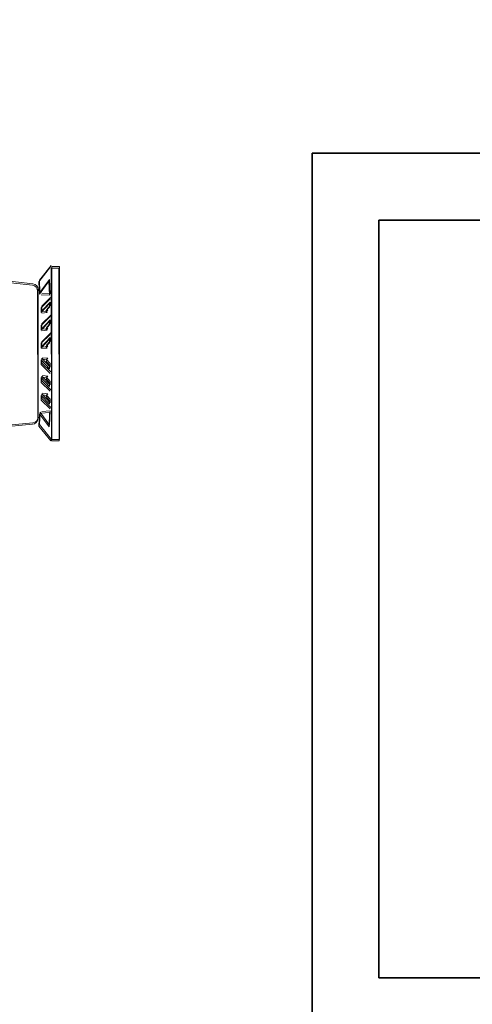
# Model space of a CAD drawing. Units: inches. Extents: x -26 to 575, y -18 to 513.
# Tile 22 of 28: x 355 to 385, y 241 to 307. Entities that reach past the tile are written whole.
import ezdxf

# ---------------------------------------------------------------- set-up
doc = ezdxf.new("R2010")
doc.units = ezdxf.units.IN
doc.header["$MEASUREMENT"] = 0
for name, color, linetype, lineweight in [('A-ANNO-DIMS', 2, 'Continuous', 18), ('A-WALL', 7, 'Continuous', 35), ('Furniture', 8, 'Continuous', 15)]:
    doc.layers.add(name, color=color, linetype=linetype, lineweight=lineweight)
doc.styles.get("Standard").update_dxf_attribs({"font": 'arial.ttf', "height": 6})
doc.dimstyles.get("Standard").update_dxf_attribs({"dimtxt": 6, "dimasz": 0.18, "dimexe": 0.18, "dimexo": 0.0625, "dimgap": 0.09, "dimtad": 0, "dimtih": 1, "dimtoh": 1, "dimzin": 0, "dimdsep": 46, "dimlunit": 3, "dimtxsty": 'Standard', "dimcen": 0.09, "dimadec": 0, "dimazin": 0, "dimtfac": 1, "dimtofl": 0, "dimtmove": 0, "dimatfit": 3, "dimfxl": 1, "dimtolj": 1, "dimtzin": 0, "dimarcsym": 0})

# ---------------------------------------------------------------- blocks, each defined once
blk = doc.blocks.new('DINING-SET-6-SEAT')
for p, q in [((16.828, 40.76, -3.573), (16.828, 41.278, -3.573)), ((16.828, 41.278, -3.573), (28.461, 41.278, -3.573)), ((16.931, 40.798, -3.573), (16.931, 41.316, -3.573)), ((16.931, 41.316, -3.573), (28.564, 41.316, -3.573)), ((28.461, 41.278, -3.573), (28.461, 40.76, -3.573)), ((28.564, 41.316, -3.573), (28.564, 40.798, -3.573)), ((47.187, 41.329, -3.573), (35.554, 41.319, -3.573)), ((35.554, 41.319, -3.573), (35.554, 40.801, -3.573)), ((47.29, 41.291, -3.573), (35.657, 41.281, -3.573)), ((35.657, 41.281, -3.573), (35.657, 40.763, -3.573)), ((47.188, 40.811, -3.573), (47.187, 41.329, -3.573)), ((47.29, 40.774, -3.573), (47.29, 41.291, -3.573)), ((28.461, 40.76, -3.573), (16.828, 40.76, -3.573)), ((16.828, 40.72, -3.573), (17.824, 39.924, -3.573)), ((28.564, 40.798, -3.573), (16.931, 40.798, -3.573)), ((16.931, 40.758, -3.573), (17.927, 39.962, -3.573)), ((17.784, 40.601, -3.573), (18.74, 40.641, -3.573)), ((18.661, 39.964, -3.573), (17.784, 40.601, -3.573)), ((17.887, 40.639, -3.573), (18.843, 40.679, -3.573)), ((18.763, 40.002, -3.573), (17.887, 40.639, -3.573)), ((18.74, 40.641, -3.573), (18.7, 40.083, -3.573)), ((18.843, 40.679, -3.573), (18.803, 40.121, -3.573)), ((18.979, 40.681, -3.573), (19.577, 40.083, -3.573)), ((19.082, 40.718, -3.573), (19.68, 40.121, -3.573)), ((19.896, 40.083, -3.573), (19.298, 40.641, -3.573)), ((19.298, 40.641, -3.573), (19.537, 40.641, -3.573)), ((19.998, 40.121, -3.573), (19.401, 40.679, -3.573)), ((19.401, 40.679, -3.573), (19.64, 40.679, -3.573)), ((19.537, 40.641, -3.573), (19.816, 40.402, -3.573)), ((19.64, 40.679, -3.573), (19.919, 40.44, -3.573)), ((19.816, 40.402, -3.573), (19.896, 40.481, -3.573)), ((19.896, 40.481, -3.573), (19.936, 40.123, -3.573)), ((19.919, 40.44, -3.573), (19.998, 40.519, -3.573)), ((19.998, 40.519, -3.573), (20.038, 40.161, -3.573)), ((20.175, 40.681, -3.573), (20.772, 40.083, -3.573)), ((20.277, 40.718, -3.573), (20.875, 40.121, -3.573)), ((21.091, 40.083, -3.573), (20.493, 40.641, -3.573)), ((20.493, 40.641, -3.573), (20.732, 40.641, -3.573)), ((21.194, 40.121, -3.573), (20.596, 40.679, -3.573)), ((20.596, 40.679, -3.573), (20.835, 40.679, -3.573)), ((20.732, 40.641, -3.573), (21.011, 40.402, -3.573)), ((20.835, 40.679, -3.573), (21.114, 40.44, -3.573)), ((21.011, 40.402, -3.573), (21.091, 40.481, -3.573)), ((21.091, 40.481, -3.573), (21.131, 40.123, -3.573)), ((21.114, 40.44, -3.573), (21.194, 40.519, -3.573)), ((21.194, 40.519, -3.573), (21.233, 40.161, -3.573)), ((21.37, 40.681, -3.573), (21.967, 40.083, -3.573)), ((21.473, 40.718, -3.573), (22.07, 40.121, -3.573)), ((22.286, 40.083, -3.573), (21.688, 40.641, -3.573)), ((21.688, 40.641, -3.573), (21.928, 40.641, -3.573)), ((22.389, 40.121, -3.573), (21.791, 40.679, -3.573)), ((21.791, 40.679, -3.573), (22.03, 40.679, -3.573)), ((21.928, 40.641, -3.573), (22.206, 40.402, -3.573)), ((22.03, 40.679, -3.573), (22.309, 40.44, -3.573)), ((22.206, 40.402, -3.573), (22.286, 40.481, -3.573)), ((22.286, 40.481, -3.573), (22.326, 40.123, -3.573)), ((22.309, 40.44, -3.573), (22.389, 40.519, -3.573)), ((22.389, 40.519, -3.573), (22.429, 40.161, -3.573)), ((23.083, 40.481, -3.573), (23.043, 40.123, -3.573)), ((23.083, 40.083, -3.573), (23.681, 40.641, -3.573)), ((23.163, 40.402, -3.573), (23.083, 40.481, -3.573)), ((23.186, 40.519, -3.573), (23.146, 40.161, -3.573)), ((23.441, 40.641, -3.573), (23.163, 40.402, -3.573)), ((23.186, 40.121, -3.573), (23.783, 40.679, -3.573)), ((23.265, 40.44, -3.573), (23.186, 40.519, -3.573)), ((23.544, 40.679, -3.573), (23.265, 40.44, -3.573)), ((23.999, 40.681, -3.573), (23.402, 40.083, -3.573)), ((23.681, 40.641, -3.573), (23.441, 40.641, -3.573)), ((24.102, 40.718, -3.573), (23.504, 40.121, -3.573)), ((23.783, 40.679, -3.573), (23.544, 40.679, -3.573)), ((24.278, 40.481, -3.573), (24.238, 40.123, -3.573)), ((24.278, 40.083, -3.573), (24.876, 40.641, -3.573)), ((24.358, 40.402, -3.573), (24.278, 40.481, -3.573)), ((24.381, 40.519, -3.573), (24.341, 40.161, -3.573)), ((24.637, 40.641, -3.573), (24.358, 40.402, -3.573)), ((24.381, 40.121, -3.573), (24.978, 40.679, -3.573)), ((24.461, 40.44, -3.573), (24.381, 40.519, -3.573)), ((24.739, 40.679, -3.573), (24.461, 40.44, -3.573)), ((25.194, 40.681, -3.573), (24.597, 40.083, -3.573)), ((24.876, 40.641, -3.573), (24.637, 40.641, -3.573)), ((25.297, 40.718, -3.573), (24.7, 40.121, -3.573)), ((24.978, 40.679, -3.573), (24.739, 40.679, -3.573)), ((25.473, 40.481, -3.573), (25.434, 40.123, -3.573)), ((25.473, 40.083, -3.573), (26.071, 40.641, -3.573)), ((25.553, 40.402, -3.573), (25.473, 40.481, -3.573)), ((25.576, 40.519, -3.573), (25.536, 40.161, -3.573)), ((25.832, 40.641, -3.573), (25.553, 40.402, -3.573)), ((25.576, 40.121, -3.573), (26.174, 40.679, -3.573)), ((25.656, 40.44, -3.573), (25.576, 40.519, -3.573)), ((25.935, 40.679, -3.573), (25.656, 40.44, -3.573)), ((26.39, 40.681, -3.573), (25.792, 40.083, -3.573)), ((26.071, 40.641, -3.573), (25.832, 40.641, -3.573)), ((26.492, 40.718, -3.573), (25.895, 40.121, -3.573)), ((26.174, 40.679, -3.573), (25.935, 40.679, -3.573)), ((27.585, 40.601, -3.573), (26.629, 40.641, -3.573)), ((26.629, 40.641, -3.573), (26.669, 40.083, -3.573)), ((26.708, 39.964, -3.573), (27.585, 40.601, -3.573)), ((27.688, 40.639, -3.573), (26.731, 40.679, -3.573)), ((26.731, 40.679, -3.573), (26.771, 40.121, -3.573)), ((26.811, 40.002, -3.573), (27.688, 40.639, -3.573)), ((28.541, 40.72, -3.573), (27.545, 39.924, -3.573)), ((28.644, 40.758, -3.573), (27.648, 39.962, -3.573)), ((35.475, 40.761, -3.573), (36.471, 39.966, -3.573)), ((35.554, 40.801, -3.573), (47.188, 40.811, -3.573)), ((35.577, 40.723, -3.573), (36.574, 39.928, -3.573)), ((35.657, 40.763, -3.573), (47.29, 40.774, -3.573)), ((36.431, 40.643, -3.573), (37.387, 40.683, -3.573)), ((37.308, 40.006, -3.573), (36.431, 40.643, -3.573)), ((36.534, 40.605, -3.573), (37.49, 40.646, -3.573)), ((37.411, 39.968, -3.573), (36.534, 40.605, -3.573)), ((37.387, 40.683, -3.573), (37.348, 40.126, -3.573)), ((37.49, 40.646, -3.573), (37.45, 40.088, -3.573)), ((37.626, 40.723, -3.573), (38.224, 40.127, -3.573)), ((37.729, 40.686, -3.573), (38.327, 40.089, -3.573)), ((38.543, 40.127, -3.573), (37.945, 40.684, -3.573)), ((37.945, 40.684, -3.573), (38.184, 40.684, -3.573)), ((38.646, 40.089, -3.573), (38.048, 40.646, -3.573)), ((38.048, 40.646, -3.573), (38.287, 40.646, -3.573)), ((38.184, 40.684, -3.573), (38.463, 40.445, -3.573)), ((38.287, 40.646, -3.573), (38.566, 40.408, -3.573)), ((38.463, 40.445, -3.573), (38.543, 40.525, -3.573)), ((38.543, 40.525, -3.573), (38.583, 40.167, -3.573)), ((38.566, 40.408, -3.573), (38.645, 40.487, -3.573)), ((38.645, 40.487, -3.573), (38.685, 40.129, -3.573)), ((38.821, 40.724, -3.573), (39.419, 40.128, -3.573)), ((38.924, 40.687, -3.573), (39.522, 40.09, -3.573)), ((39.738, 40.128, -3.573), (39.14, 40.685, -3.573)), ((39.14, 40.685, -3.573), (39.379, 40.685, -3.573)), ((39.841, 40.09, -3.573), (39.243, 40.647, -3.573)), ((39.243, 40.647, -3.573), (39.482, 40.647, -3.573)), ((39.379, 40.685, -3.573), (39.658, 40.446, -3.573)), ((39.482, 40.647, -3.573), (39.761, 40.409, -3.573)), ((39.658, 40.446, -3.573), (39.738, 40.526, -3.573)), ((39.738, 40.526, -3.573), (39.778, 40.168, -3.573)), ((39.761, 40.409, -3.573), (39.841, 40.488, -3.573)), ((39.841, 40.488, -3.573), (39.881, 40.13, -3.573)), ((40.016, 40.725, -3.573), (40.615, 40.129, -3.573)), ((40.119, 40.688, -3.573), (40.717, 40.091, -3.573)), ((40.933, 40.129, -3.573), (40.335, 40.686, -3.573)), ((40.335, 40.686, -3.573), (40.574, 40.686, -3.573)), ((41.036, 40.091, -3.573), (40.438, 40.648, -3.573)), ((40.438, 40.648, -3.573), (40.677, 40.648, -3.573)), ((40.574, 40.686, -3.573), (40.853, 40.447, -3.573)), ((40.677, 40.648, -3.573), (40.956, 40.41, -3.573)), ((40.853, 40.447, -3.573), (40.933, 40.527, -3.573)), ((40.933, 40.527, -3.573), (40.973, 40.169, -3.573)), ((40.956, 40.41, -3.573), (41.036, 40.489, -3.573)), ((41.036, 40.489, -3.573), (41.076, 40.131, -3.573)), ((41.73, 40.528, -3.573), (41.69, 40.169, -3.573)), ((41.73, 40.13, -3.573), (42.327, 40.688, -3.573)), ((41.81, 40.448, -3.573), (41.73, 40.528, -3.573)), ((41.833, 40.49, -3.573), (41.793, 40.132, -3.573)), ((42.088, 40.687, -3.573), (41.81, 40.448, -3.573)), ((41.833, 40.092, -3.573), (42.43, 40.65, -3.573)), ((41.912, 40.41, -3.573), (41.833, 40.49, -3.573)), ((42.191, 40.65, -3.573), (41.912, 40.41, -3.573)), ((42.646, 40.728, -3.573), (42.049, 40.13, -3.573)), ((42.327, 40.688, -3.573), (42.088, 40.687, -3.573)), ((42.749, 40.69, -3.573), (42.152, 40.092, -3.573)), ((42.43, 40.65, -3.573), (42.191, 40.65, -3.573)), ((42.925, 40.529, -3.573), (42.885, 40.17, -3.573)), ((42.925, 40.131, -3.573), (43.522, 40.689, -3.573)), ((43.005, 40.449, -3.573), (42.925, 40.529, -3.573)), ((43.028, 40.491, -3.573), (42.988, 40.133, -3.573)), ((43.283, 40.688, -3.573), (43.005, 40.449, -3.573)), ((43.028, 40.093, -3.573), (43.625, 40.651, -3.573)), ((43.108, 40.412, -3.573), (43.028, 40.491, -3.573)), ((43.386, 40.651, -3.573), (43.108, 40.412, -3.573)), ((43.841, 40.729, -3.573), (43.244, 40.131, -3.573)), ((43.522, 40.689, -3.573), (43.283, 40.688, -3.573)), ((43.944, 40.691, -3.573), (43.347, 40.093, -3.573)), ((43.625, 40.651, -3.573), (43.386, 40.651, -3.573)), ((44.12, 40.53, -3.573), (44.081, 40.171, -3.573)), ((44.2, 40.45, -3.573), (44.12, 40.53, -3.573)), ((44.121, 40.132, -3.573), (44.718, 40.69, -3.573)), ((44.223, 40.492, -3.573), (44.183, 40.134, -3.573)), ((44.479, 40.69, -3.573), (44.2, 40.45, -3.573)), ((44.223, 40.094, -3.573), (44.82, 40.652, -3.573)), ((44.303, 40.413, -3.573), (44.223, 40.492, -3.573)), ((44.581, 40.652, -3.573), (44.303, 40.413, -3.573)), ((45.036, 40.73, -3.573), (44.439, 40.132, -3.573)), ((44.718, 40.69, -3.573), (44.479, 40.69, -3.573)), ((45.139, 40.692, -3.573), (44.542, 40.094, -3.573)), ((44.82, 40.652, -3.573), (44.581, 40.652, -3.573)), ((46.232, 40.651, -3.573), (45.275, 40.69, -3.573)), ((45.275, 40.69, -3.573), (45.316, 40.133, -3.573)), ((45.356, 40.013, -3.573), (46.232, 40.651, -3.573)), ((46.334, 40.613, -3.573), (45.378, 40.652, -3.573)), ((45.378, 40.652, -3.573), (45.419, 40.095, -3.573)), ((45.458, 39.976, -3.573), (46.334, 40.613, -3.573)), ((47.188, 40.772, -3.573), (46.192, 39.974, -3.573)), ((47.29, 40.734, -3.573), (46.295, 39.936, -3.573)), ((17.824, 39.924, -3.573), (18.661, 39.964, -3.573)), ((17.927, 39.962, -3.573), (18.763, 40.002, -3.573)), ((26.909, 39.844, -3.573), (18.345, 39.844, -3.573)), ((27.012, 39.882, -3.573), (18.448, 39.882, -3.573)), ((19.577, 40.083, -3.573), (19.896, 40.083, -3.573)), ((19.68, 40.121, -3.573), (19.998, 40.121, -3.573)), ((20.772, 40.083, -3.573), (21.091, 40.083, -3.573)), ((20.875, 40.121, -3.573), (21.194, 40.121, -3.573)), ((21.967, 40.083, -3.573), (22.286, 40.083, -3.573)), ((22.07, 40.121, -3.573), (22.389, 40.121, -3.573)), ((23.402, 40.083, -3.573), (23.083, 40.083, -3.573)), ((23.504, 40.121, -3.573), (23.186, 40.121, -3.573)), ((24.597, 40.083, -3.573), (24.278, 40.083, -3.573)), ((24.7, 40.121, -3.573), (24.381, 40.121, -3.573)), ((25.792, 40.083, -3.573), (25.473, 40.083, -3.573)), ((25.895, 40.121, -3.573), (25.576, 40.121, -3.573)), ((27.545, 39.924, -3.573), (26.708, 39.964, -3.573)), ((27.648, 39.962, -3.573), (26.811, 40.002, -3.573)), ((36.471, 39.966, -3.573), (37.308, 40.006, -3.573)), ((36.574, 39.928, -3.573), (37.411, 39.968, -3.573)), ((37.107, 39.887, -3.573), (45.671, 39.894, -3.573)), ((37.21, 39.849, -3.573), (45.774, 39.856, -3.573)), ((38.224, 40.127, -3.573), (38.543, 40.127, -3.573)), ((38.327, 40.089, -3.573), (38.646, 40.089, -3.573)), ((39.419, 40.128, -3.573), (39.738, 40.128, -3.573)), ((39.522, 40.09, -3.573), (39.841, 40.09, -3.573)), ((40.615, 40.129, -3.573), (40.933, 40.129, -3.573)), ((40.717, 40.091, -3.573), (41.036, 40.091, -3.573)), ((42.049, 40.13, -3.573), (41.73, 40.13, -3.573)), ((42.152, 40.092, -3.573), (41.833, 40.092, -3.573)), ((43.244, 40.131, -3.573), (42.925, 40.131, -3.573)), ((43.347, 40.093, -3.573), (43.028, 40.093, -3.573)), ((44.439, 40.132, -3.573), (44.121, 40.132, -3.573)), ((44.542, 40.094, -3.573), (44.223, 40.094, -3.573)), ((46.192, 39.974, -3.573), (45.356, 40.013, -3.573)), ((46.295, 39.936, -3.573), (45.458, 39.976, -3.573)), ((17.949, 39.484, -3.573), (16.91, 28.653, -3.573)), ((18.052, 39.522, -3.573), (17.012, 28.691, -3.573)), ((28.493, 28.659, -3.573), (27.305, 39.489, -3.573)), ((28.595, 28.696, -3.573), (27.408, 39.527, -3.573)), ((35.534, 28.7, -3.573), (36.712, 39.531, -3.573)), ((35.636, 28.662, -3.573), (36.814, 39.494, -3.573)), ((46.068, 39.534, -3.573), (47.117, 28.704, -3.573)), ((46.171, 39.496, -3.573), (47.219, 28.667, -3.573)), ((16.194, 22.294, -1.308), (26.662, 30.717, -1.308)), ((46.474, 31.041, -1.308), (18.1, 31.041, -1.308)), ((14.74, 19.68, -1.308), (28.116, 30.426, -1.308)), ((25.79, 15.904, -1.308), (43.819, 30.136, -1.308)), ((17.306, 28.217, -3.573), (28.097, 28.217, -3.573)), ((17.409, 28.255, -3.573), (28.199, 28.255, -3.573)), ((46.72, 28.268, -3.573), (35.93, 28.258, -3.573)), ((46.823, 28.23, -3.573), (36.033, 28.22, -3.573)), ((18.1, 10.54, -1.308), (39.457, 27.522, -1.308)), ((0, 14.987, -3.573), (0.01, 26.621, -3.573)), ((0.01, 26.621, -3.573), (0.528, 26.62, -3.573)), ((0.037, 14.884, -3.573), (0.048, 26.518, -3.573)), ((0.048, 26.518, -3.573), (0.565, 26.517, -3.573)), ((0.528, 26.62, -3.573), (0.517, 14.987, -3.573)), ((0.565, 26.517, -3.573), (0.555, 14.884, -3.573)), ((0.567, 26.7, -3.573), (1.363, 25.703, -3.573)), ((0.605, 26.597, -3.573), (1.401, 25.6, -3.573)), ((12.629, 26.641, -3.573), (1.797, 25.463, -3.573)), ((12.667, 26.538, -3.573), (1.835, 25.36, -3.573)), ((52.057, 26.538, -3.573), (62.889, 25.36, -3.573)), ((52.095, 26.641, -3.573), (62.926, 25.463, -3.573)), ((64.119, 26.597, -3.573), (63.323, 25.6, -3.573)), ((64.156, 26.7, -3.573), (63.361, 25.703, -3.573)), ((64.676, 26.518, -3.573), (64.159, 26.517, -3.573)), ((64.159, 26.517, -3.573), (64.169, 14.884, -3.573)), ((64.714, 26.621, -3.573), (64.196, 26.62, -3.573)), ((64.196, 26.62, -3.573), (64.207, 14.987, -3.573)), ((64.686, 14.884, -3.573), (64.676, 26.518, -3.573)), ((64.724, 14.987, -3.573), (64.714, 26.621, -3.573)), ((13.061, 15.454, -3.573), (13.071, 26.244, -3.573)), ((13.099, 15.351, -3.573), (13.108, 26.142, -3.573)), ((51.625, 15.351, -3.573), (51.615, 26.142, -3.573)), ((51.663, 15.454, -3.573), (51.653, 26.244, -3.573)), ((0.686, 25.744, -3.573), (0.645, 24.787, -3.573)), ((0.724, 25.641, -3.573), (0.683, 24.685, -3.573)), ((1.322, 24.866, -3.573), (0.686, 25.744, -3.573)), ((1.36, 24.764, -3.573), (0.724, 25.641, -3.573)), ((1.363, 25.703, -3.573), (1.322, 24.866, -3.573)), ((1.401, 25.6, -3.573), (1.36, 24.764, -3.573)), ((63.323, 25.6, -3.573), (63.364, 24.764, -3.573)), ((63.361, 25.703, -3.573), (63.401, 24.866, -3.573)), ((63.364, 24.764, -3.573), (64, 25.641, -3.573)), ((63.401, 24.866, -3.573), (64.038, 25.744, -3.573)), ((64, 25.641, -3.573), (64.041, 24.685, -3.573)), ((64.038, 25.744, -3.573), (64.078, 24.787, -3.573)), ((0.605, 24.548, -3.573), (1.202, 23.95, -3.573)), ((0.645, 24.787, -3.573), (1.203, 24.827, -3.573)), ((0.683, 24.685, -3.573), (1.241, 24.724, -3.573)), ((1.442, 25.067, -3.573), (1.435, 16.503, -3.573)), ((1.48, 24.964, -3.573), (1.472, 16.401, -3.573)), ((63.244, 24.964, -3.573), (63.252, 16.401, -3.573)), ((63.282, 25.067, -3.573), (63.289, 16.503, -3.573)), ((64.041, 24.685, -3.573), (63.483, 24.724, -3.573)), ((64.078, 24.787, -3.573), (63.521, 24.827, -3.573)), ((64.118, 24.548, -3.573), (63.522, 23.95, -3.573)), ((0.643, 24.446, -3.573), (1.24, 23.847, -3.573)), ((1.202, 23.632, -3.573), (0.645, 24.23, -3.573)), ((0.645, 24.23, -3.573), (0.645, 23.991, -3.573)), ((0.645, 23.991, -3.573), (0.883, 23.712, -3.573)), ((0.683, 24.127, -3.573), (0.682, 23.888, -3.573)), ((0.682, 23.888, -3.573), (0.921, 23.609, -3.573)), ((1.24, 23.529, -3.573), (0.683, 24.127, -3.573)), ((1.202, 23.95, -3.573), (1.202, 23.632, -3.573)), ((40.039, 15.033, -1.308), (51.38, 24.327, -1.308)), ((64.081, 24.446, -3.573), (63.484, 23.847, -3.573)), ((63.484, 23.529, -3.573), (64.041, 24.127, -3.573)), ((63.522, 23.632, -3.573), (64.079, 24.23, -3.573)), ((63.522, 23.95, -3.573), (63.522, 23.632, -3.573)), ((64.041, 23.888, -3.573), (63.803, 23.609, -3.573)), ((64.079, 23.991, -3.573), (63.84, 23.712, -3.573)), ((64.041, 24.127, -3.573), (64.041, 23.888, -3.573)), ((64.079, 24.23, -3.573), (64.079, 23.991, -3.573)), ((0.604, 23.353, -3.573), (1.201, 22.755, -3.573)), ((0.642, 23.25, -3.573), (1.239, 22.652, -3.573)), ((0.883, 23.712, -3.573), (0.804, 23.632, -3.573)), ((0.804, 23.632, -3.573), (1.162, 23.592, -3.573)), ((0.921, 23.609, -3.573), (0.841, 23.529, -3.573)), ((0.841, 23.529, -3.573), (1.2, 23.489, -3.573)), ((1.24, 23.847, -3.573), (1.24, 23.529, -3.573)), ((63.484, 23.847, -3.573), (63.484, 23.529, -3.573)), ((64.082, 23.25, -3.573), (63.485, 22.652, -3.573)), ((64.12, 23.353, -3.573), (63.523, 22.755, -3.573)), ((63.882, 23.529, -3.573), (63.524, 23.489, -3.573)), ((63.92, 23.632, -3.573), (63.562, 23.592, -3.573)), ((63.803, 23.609, -3.573), (63.882, 23.529, -3.573)), ((63.84, 23.712, -3.573), (63.92, 23.632, -3.573)), ((1.201, 22.436, -3.573), (0.644, 23.034, -3.573)), ((0.644, 23.034, -3.573), (0.644, 22.795, -3.573)), ((0.644, 22.795, -3.573), (0.882, 22.516, -3.573)), ((0.682, 22.932, -3.573), (0.681, 22.693, -3.573)), ((0.681, 22.693, -3.573), (0.92, 22.414, -3.573)), ((1.239, 22.334, -3.573), (0.682, 22.932, -3.573)), ((1.201, 22.755, -3.573), (1.201, 22.436, -3.573)), ((1.239, 22.652, -3.573), (1.239, 22.334, -3.573)), ((63.485, 22.334, -3.573), (64.042, 22.932, -3.573)), ((63.485, 22.652, -3.573), (63.485, 22.334, -3.573)), ((63.523, 22.436, -3.573), (64.08, 23.034, -3.573)), ((63.523, 22.755, -3.573), (63.523, 22.436, -3.573)), ((64.042, 22.693, -3.573), (63.804, 22.414, -3.573)), ((64.08, 22.795, -3.573), (63.842, 22.516, -3.573)), ((64.042, 22.932, -3.573), (64.042, 22.693, -3.573)), ((64.08, 23.034, -3.573), (64.08, 22.795, -3.573)), ((0.603, 22.158, -3.573), (1.2, 21.56, -3.573)), ((0.641, 22.055, -3.573), (1.238, 21.457, -3.573)), ((0.882, 22.516, -3.573), (0.803, 22.437, -3.573)), ((0.803, 22.437, -3.573), (1.161, 22.397, -3.573)), ((0.92, 22.414, -3.573), (0.84, 22.334, -3.573)), ((0.84, 22.334, -3.573), (1.199, 22.294, -3.573)), ((64.083, 22.055, -3.573), (63.486, 21.457, -3.573)), ((64.121, 22.158, -3.573), (63.524, 21.56, -3.573)), ((63.883, 22.334, -3.573), (63.525, 22.294, -3.573)), ((63.921, 22.437, -3.573), (63.563, 22.397, -3.573)), ((63.804, 22.414, -3.573), (63.883, 22.334, -3.573)), ((63.842, 22.516, -3.573), (63.921, 22.437, -3.573)), ((1.2, 21.241, -3.573), (0.643, 21.839, -3.573)), ((0.643, 21.839, -3.573), (0.643, 21.6, -3.573)), ((0.643, 21.6, -3.573), (0.881, 21.321, -3.573)), ((0.681, 21.736, -3.573), (0.68, 21.497, -3.573)), ((0.68, 21.497, -3.573), (0.919, 21.218, -3.573)), ((1.238, 21.138, -3.573), (0.681, 21.736, -3.573)), ((0.881, 21.321, -3.573), (0.802, 21.241, -3.573)), ((0.802, 21.241, -3.573), (1.16, 21.201, -3.573)), ((0.919, 21.218, -3.573), (0.839, 21.139, -3.573)), ((1.2, 21.56, -3.573), (1.2, 21.241, -3.573)), ((1.238, 21.457, -3.573), (1.238, 21.138, -3.573)), ((63.486, 21.138, -3.573), (64.043, 21.736, -3.573)), ((63.486, 21.457, -3.573), (63.486, 21.138, -3.573)), ((63.524, 21.241, -3.573), (64.081, 21.839, -3.573)), ((63.524, 21.56, -3.573), (63.524, 21.241, -3.573)), ((63.922, 21.241, -3.573), (63.564, 21.201, -3.573)), ((64.043, 21.497, -3.573), (63.805, 21.218, -3.573)), ((63.805, 21.218, -3.573), (63.884, 21.139, -3.573)), ((64.081, 21.6, -3.573), (63.843, 21.321, -3.573)), ((63.843, 21.321, -3.573), (63.922, 21.241, -3.573)), ((64.043, 21.736, -3.573), (64.043, 21.497, -3.573)), ((64.081, 21.839, -3.573), (64.081, 21.6, -3.573)), ((0.839, 21.139, -3.573), (1.198, 21.099, -3.573)), ((63.884, 21.139, -3.573), (63.526, 21.099, -3.573)), ((0.601, 19.529, -3.573), (1.199, 20.126, -3.573)), ((0.639, 19.426, -3.573), (1.237, 20.023, -3.573)), ((1.199, 20.444, -3.573), (0.641, 19.847, -3.573)), ((0.641, 20.086, -3.573), (0.88, 20.365, -3.573)), ((0.641, 19.847, -3.573), (0.641, 20.086, -3.573)), ((1.237, 20.342, -3.573), (0.679, 19.744, -3.573)), ((0.679, 19.983, -3.573), (0.918, 20.262, -3.573)), ((0.679, 19.744, -3.573), (0.679, 19.983, -3.573)), ((0.801, 20.445, -3.573), (1.159, 20.484, -3.573)), ((0.88, 20.365, -3.573), (0.801, 20.445, -3.573)), ((0.839, 20.342, -3.573), (1.197, 20.381, -3.573)), ((0.918, 20.262, -3.573), (0.839, 20.342, -3.573)), ((1.199, 20.126, -3.573), (1.199, 20.444, -3.573)), ((1.237, 20.023, -3.573), (1.237, 20.342, -3.573)), ((34.805, 10.386, -1.308), (47.018, 19.971, -1.308)), ((63.487, 20.023, -3.573), (63.487, 20.342, -3.573)), ((63.487, 20.342, -3.573), (64.045, 19.744, -3.573)), ((64.085, 19.426, -3.573), (63.487, 20.023, -3.573)), ((63.525, 20.126, -3.573), (63.525, 20.444, -3.573)), ((63.525, 20.444, -3.573), (64.083, 19.847, -3.573)), ((64.123, 19.529, -3.573), (63.525, 20.126, -3.573)), ((63.885, 20.342, -3.573), (63.527, 20.381, -3.573)), ((63.923, 20.445, -3.573), (63.565, 20.484, -3.573)), ((63.806, 20.262, -3.573), (63.885, 20.342, -3.573)), ((64.045, 19.983, -3.573), (63.806, 20.262, -3.573)), ((63.843, 20.365, -3.573), (63.923, 20.445, -3.573)), ((64.083, 20.086, -3.573), (63.843, 20.365, -3.573)), ((64.045, 19.744, -3.573), (64.045, 19.983, -3.573)), ((64.083, 19.847, -3.573), (64.083, 20.086, -3.573)), ((1.198, 19.249, -3.573), (0.64, 18.652, -3.573)), ((0.8, 19.249, -3.573), (1.158, 19.289, -3.573)), ((0.879, 19.17, -3.573), (0.8, 19.249, -3.573)), ((1.198, 18.93, -3.573), (1.198, 19.249, -3.573)), ((63.526, 18.93, -3.573), (63.526, 19.249, -3.573)), ((63.526, 19.249, -3.573), (64.084, 18.652, -3.573)), ((63.924, 19.249, -3.573), (63.566, 19.289, -3.573)), ((63.844, 19.17, -3.573), (63.924, 19.249, -3.573)), ((0.6, 18.333, -3.573), (1.198, 18.93, -3.573)), ((0.638, 18.231, -3.573), (1.236, 18.828, -3.573)), ((0.64, 18.891, -3.573), (0.879, 19.17, -3.573)), ((0.64, 18.652, -3.573), (0.64, 18.891, -3.573)), ((1.236, 19.146, -3.573), (0.678, 18.549, -3.573)), ((0.678, 18.788, -3.573), (0.917, 19.067, -3.573)), ((0.678, 18.549, -3.573), (0.678, 18.788, -3.573)), ((0.838, 19.147, -3.573), (1.196, 19.186, -3.573)), ((0.917, 19.067, -3.573), (0.838, 19.147, -3.573)), ((1.236, 18.828, -3.573), (1.236, 19.146, -3.573)), ((63.488, 18.828, -3.573), (63.488, 19.146, -3.573)), ((63.488, 19.146, -3.573), (64.046, 18.549, -3.573)), ((64.086, 18.231, -3.573), (63.488, 18.828, -3.573)), ((64.124, 18.333, -3.573), (63.526, 18.93, -3.573)), ((63.886, 19.147, -3.573), (63.528, 19.186, -3.573)), ((63.807, 19.067, -3.573), (63.886, 19.147, -3.573)), ((64.046, 18.788, -3.573), (63.807, 19.067, -3.573)), ((64.084, 18.891, -3.573), (63.844, 19.17, -3.573)), ((64.046, 18.549, -3.573), (64.046, 18.788, -3.573)), ((64.084, 18.652, -3.573), (64.084, 18.891, -3.573)), ((1.197, 18.054, -3.573), (0.639, 17.457, -3.573)), ((0.639, 17.696, -3.573), (0.878, 17.974, -3.573)), ((1.235, 17.951, -3.573), (0.677, 17.354, -3.573)), ((0.799, 18.054, -3.573), (1.157, 18.094, -3.573)), ((0.878, 17.974, -3.573), (0.799, 18.054, -3.573)), ((0.837, 17.951, -3.573), (1.195, 17.991, -3.573)), ((0.916, 17.872, -3.573), (0.837, 17.951, -3.573)), ((1.197, 17.735, -3.573), (1.197, 18.054, -3.573)), ((1.234, 17.632, -3.573), (1.235, 17.951, -3.573)), ((63.489, 17.632, -3.573), (63.489, 17.951, -3.573)), ((63.489, 17.951, -3.573), (64.047, 17.354, -3.573)), ((63.527, 17.735, -3.573), (63.527, 18.054, -3.573)), ((63.527, 18.054, -3.573), (64.085, 17.457, -3.573)), ((63.887, 17.951, -3.573), (63.529, 17.991, -3.573)), ((63.925, 18.054, -3.573), (63.567, 18.094, -3.573)), ((63.808, 17.872, -3.573), (63.887, 17.951, -3.573)), ((63.846, 17.974, -3.573), (63.925, 18.054, -3.573)), ((64.085, 17.696, -3.573), (63.846, 17.974, -3.573)), ((0.599, 17.138, -3.573), (1.197, 17.735, -3.573)), ((0.637, 17.035, -3.573), (1.234, 17.632, -3.573)), ((0.639, 17.457, -3.573), (0.639, 17.696, -3.573)), ((0.677, 17.593, -3.573), (0.916, 17.872, -3.573)), ((0.677, 17.354, -3.573), (0.677, 17.593, -3.573)), ((64.087, 17.035, -3.573), (63.489, 17.632, -3.573)), ((64.125, 17.138, -3.573), (63.527, 17.735, -3.573)), ((64.047, 17.593, -3.573), (63.808, 17.872, -3.573)), ((64.047, 17.354, -3.573), (64.047, 17.593, -3.573)), ((64.085, 17.457, -3.573), (64.085, 17.696, -3.573)), ((0.677, 15.943, -3.573), (0.639, 16.899, -3.573)), ((0.639, 16.899, -3.573), (1.196, 16.859, -3.573)), ((0.715, 15.84, -3.573), (0.676, 16.796, -3.573)), ((0.676, 16.796, -3.573), (1.234, 16.756, -3.573)), ((1.315, 16.819, -3.573), (0.677, 15.943, -3.573)), ((1.353, 16.716, -3.573), (0.715, 15.84, -3.573)), ((1.354, 15.982, -3.573), (1.315, 16.819, -3.573)), ((1.392, 15.879, -3.573), (1.353, 16.716, -3.573)), ((63.332, 15.879, -3.573), (63.371, 16.716, -3.573)), ((63.369, 15.982, -3.573), (63.408, 16.819, -3.573)), ((63.371, 16.716, -3.573), (64.009, 15.84, -3.573)), ((63.408, 16.819, -3.573), (64.046, 15.943, -3.573)), ((64.048, 16.796, -3.573), (63.49, 16.756, -3.573)), ((64.085, 16.899, -3.573), (63.528, 16.859, -3.573)), ((64.009, 15.84, -3.573), (64.048, 16.796, -3.573)), ((64.046, 15.943, -3.573), (64.085, 16.899, -3.573)), ((0.557, 14.987, -3.573), (1.354, 15.982, -3.573)), ((1.795, 16.106, -3.573), (12.624, 15.058, -3.573)), ((1.832, 16.004, -3.573), (12.662, 14.955, -3.573)), ((62.892, 16.004, -3.573), (52.062, 14.955, -3.573)), ((62.929, 16.106, -3.573), (52.099, 15.058, -3.573)), ((64.167, 14.987, -3.573), (63.369, 15.982, -3.573)), ((0.595, 14.884, -3.573), (1.392, 15.879, -3.573)), ((64.129, 14.884, -3.573), (63.332, 15.879, -3.573)), ((0.517, 14.987, -3.573), (0, 14.987, -3.573)), ((0.555, 14.884, -3.573), (0.037, 14.884, -3.573)), ((64.169, 14.884, -3.573), (64.686, 14.884, -3.573)), ((64.207, 14.987, -3.573), (64.724, 14.987, -3.573)), ((17.949, 1.845, -3.573), (16.91, 12.676, -3.573)), ((18.052, 1.807, -3.573), (17.012, 12.638, -3.573)), ((17.306, 13.113, -3.573), (28.097, 13.113, -3.573)), ((17.409, 13.075, -3.573), (28.199, 13.075, -3.573)), ((28.493, 12.671, -3.573), (27.305, 1.84, -3.573)), ((28.595, 12.633, -3.573), (27.408, 1.802, -3.573)), ((35.534, 12.63, -3.573), (36.712, 1.798, -3.573)), ((35.636, 12.668, -3.573), (36.814, 1.836, -3.573)), ((46.72, 13.062, -3.573), (35.93, 13.071, -3.573)), ((46.823, 13.1, -3.573), (36.033, 13.109, -3.573)), ((46.068, 1.795, -3.573), (47.117, 12.625, -3.573)), ((46.171, 1.833, -3.573), (47.219, 12.663, -3.573)), ((18.1, 10.54, -1.308), (46.474, 10.54, -1.308)), ((16.828, 0.609, -3.573), (17.824, 1.405, -3.573)), ((16.931, 0.571, -3.573), (17.927, 1.367, -3.573)), ((18.661, 1.366, -3.573), (17.784, 0.728, -3.573)), ((17.824, 1.405, -3.573), (18.661, 1.366, -3.573)), ((18.763, 1.328, -3.573), (17.887, 0.691, -3.573)), ((17.927, 1.367, -3.573), (18.763, 1.328, -3.573)), ((26.909, 1.485, -3.573), (18.345, 1.485, -3.573)), ((27.012, 1.447, -3.573), (18.448, 1.447, -3.573)), ((27.545, 1.405, -3.573), (26.708, 1.366, -3.573)), ((26.708, 1.366, -3.573), (27.585, 0.728, -3.573)), ((27.648, 1.367, -3.573), (26.811, 1.328, -3.573)), ((26.811, 1.328, -3.573), (27.688, 0.691, -3.573)), ((28.541, 0.609, -3.573), (27.545, 1.405, -3.573)), ((28.644, 0.571, -3.573), (27.648, 1.367, -3.573)), ((35.475, 0.568, -3.573), (36.471, 1.364, -3.573)), ((35.577, 0.606, -3.573), (36.574, 1.401, -3.573)), ((36.471, 1.364, -3.573), (37.308, 1.323, -3.573)), ((37.411, 1.361, -3.573), (36.534, 0.724, -3.573)), ((36.574, 1.401, -3.573), (37.411, 1.361, -3.573)), ((37.107, 1.443, -3.573), (45.671, 1.435, -3.573)), ((37.21, 1.48, -3.573), (45.774, 1.473, -3.573)), ((46.192, 1.355, -3.573), (45.356, 1.316, -3.573)), ((46.295, 1.393, -3.573), (45.458, 1.354, -3.573)), ((45.458, 1.354, -3.573), (46.334, 0.716, -3.573)), ((47.188, 0.558, -3.573), (46.192, 1.355, -3.573)), ((47.29, 0.596, -3.573), (46.295, 1.393, -3.573)), ((17.784, 0.728, -3.573), (18.74, 0.689, -3.573)), ((17.887, 0.691, -3.573), (18.843, 0.651, -3.573)), ((18.74, 0.689, -3.573), (18.7, 1.246, -3.573)), ((18.843, 0.651, -3.573), (18.803, 1.208, -3.573)), ((18.979, 0.649, -3.573), (19.577, 1.246, -3.573)), ((19.082, 0.611, -3.573), (19.68, 1.208, -3.573)), ((19.896, 1.246, -3.573), (19.298, 0.689, -3.573)), ((19.298, 0.689, -3.573), (19.537, 0.689, -3.573)), ((19.998, 1.208, -3.573), (19.401, 0.651, -3.573)), ((19.537, 0.689, -3.573), (19.816, 0.928, -3.573)), ((19.577, 1.246, -3.573), (19.896, 1.246, -3.573)), ((19.64, 0.651, -3.573), (19.919, 0.89, -3.573)), ((19.68, 1.208, -3.573), (19.998, 1.208, -3.573)), ((19.816, 0.928, -3.573), (19.896, 0.848, -3.573)), ((19.896, 0.848, -3.573), (19.936, 1.206, -3.573)), ((19.919, 0.89, -3.573), (19.998, 0.81, -3.573)), ((19.998, 0.81, -3.573), (20.038, 1.168, -3.573)), ((20.175, 0.649, -3.573), (20.772, 1.246, -3.573)), ((20.277, 0.611, -3.573), (20.875, 1.208, -3.573)), ((21.091, 1.246, -3.573), (20.493, 0.689, -3.573)), ((20.493, 0.689, -3.573), (20.732, 0.689, -3.573)), ((21.194, 1.208, -3.573), (20.596, 0.651, -3.573)), ((20.732, 0.689, -3.573), (21.011, 0.928, -3.573)), ((20.772, 1.246, -3.573), (21.091, 1.246, -3.573)), ((20.835, 0.651, -3.573), (21.114, 0.89, -3.573)), ((20.875, 1.208, -3.573), (21.194, 1.208, -3.573)), ((21.011, 0.928, -3.573), (21.091, 0.848, -3.573)), ((21.091, 0.848, -3.573), (21.131, 1.206, -3.573)), ((21.114, 0.89, -3.573), (21.194, 0.81, -3.573)), ((21.194, 0.81, -3.573), (21.233, 1.168, -3.573)), ((21.37, 0.649, -3.573), (21.967, 1.246, -3.573)), ((21.473, 0.611, -3.573), (22.07, 1.208, -3.573)), ((22.286, 1.246, -3.573), (21.688, 0.689, -3.573)), ((21.688, 0.689, -3.573), (21.928, 0.689, -3.573)), ((22.389, 1.208, -3.573), (21.791, 0.651, -3.573)), ((21.928, 0.689, -3.573), (22.206, 0.928, -3.573)), ((21.967, 1.246, -3.573), (22.286, 1.246, -3.573)), ((22.03, 0.651, -3.573), (22.309, 0.89, -3.573)), ((22.07, 1.208, -3.573), (22.389, 1.208, -3.573)), ((22.206, 0.928, -3.573), (22.286, 0.848, -3.573)), ((22.286, 0.848, -3.573), (22.326, 1.206, -3.573)), ((22.309, 0.89, -3.573), (22.389, 0.81, -3.573)), ((22.389, 0.81, -3.573), (22.429, 1.168, -3.573)), ((23.083, 0.848, -3.573), (23.043, 1.206, -3.573)), ((23.402, 1.246, -3.573), (23.083, 1.246, -3.573)), ((23.083, 1.246, -3.573), (23.681, 0.689, -3.573)), ((23.163, 0.928, -3.573), (23.083, 0.848, -3.573)), ((23.186, 0.81, -3.573), (23.146, 1.168, -3.573)), ((23.441, 0.689, -3.573), (23.163, 0.928, -3.573)), ((23.504, 1.208, -3.573), (23.186, 1.208, -3.573)), ((23.186, 1.208, -3.573), (23.783, 0.651, -3.573)), ((23.265, 0.89, -3.573), (23.186, 0.81, -3.573)), ((23.544, 0.651, -3.573), (23.265, 0.89, -3.573)), ((23.999, 0.649, -3.573), (23.402, 1.246, -3.573)), ((23.681, 0.689, -3.573), (23.441, 0.689, -3.573)), ((24.102, 0.611, -3.573), (23.504, 1.208, -3.573)), ((24.278, 0.848, -3.573), (24.238, 1.206, -3.573)), ((24.597, 1.246, -3.573), (24.278, 1.246, -3.573)), ((24.278, 1.246, -3.573), (24.876, 0.689, -3.573)), ((24.358, 0.928, -3.573), (24.278, 0.848, -3.573)), ((24.381, 0.81, -3.573), (24.341, 1.168, -3.573)), ((24.637, 0.689, -3.573), (24.358, 0.928, -3.573)), ((24.7, 1.208, -3.573), (24.381, 1.208, -3.573)), ((24.381, 1.208, -3.573), (24.978, 0.651, -3.573)), ((24.461, 0.89, -3.573), (24.381, 0.81, -3.573)), ((24.739, 0.651, -3.573), (24.461, 0.89, -3.573)), ((25.194, 0.649, -3.573), (24.597, 1.246, -3.573)), ((24.876, 0.689, -3.573), (24.637, 0.689, -3.573)), ((25.297, 0.611, -3.573), (24.7, 1.208, -3.573)), ((25.473, 0.848, -3.573), (25.434, 1.206, -3.573)), ((25.792, 1.246, -3.573), (25.473, 1.246, -3.573)), ((25.473, 1.246, -3.573), (26.071, 0.689, -3.573)), ((25.553, 0.928, -3.573), (25.473, 0.848, -3.573)), ((25.576, 0.81, -3.573), (25.536, 1.168, -3.573)), ((25.832, 0.689, -3.573), (25.553, 0.928, -3.573)), ((25.895, 1.208, -3.573), (25.576, 1.208, -3.573)), ((25.576, 1.208, -3.573), (26.174, 0.651, -3.573)), ((25.656, 0.89, -3.573), (25.576, 0.81, -3.573)), ((25.935, 0.651, -3.573), (25.656, 0.89, -3.573)), ((26.39, 0.649, -3.573), (25.792, 1.246, -3.573)), ((26.071, 0.689, -3.573), (25.832, 0.689, -3.573)), ((26.492, 0.611, -3.573), (25.895, 1.208, -3.573)), ((26.629, 0.689, -3.573), (26.669, 1.246, -3.573)), ((27.585, 0.728, -3.573), (26.629, 0.689, -3.573)), ((26.731, 0.651, -3.573), (26.771, 1.208, -3.573)), ((27.688, 0.691, -3.573), (26.731, 0.651, -3.573)), ((37.308, 1.323, -3.573), (36.431, 0.687, -3.573)), ((36.431, 0.687, -3.573), (37.387, 0.646, -3.573)), ((36.534, 0.724, -3.573), (37.49, 0.684, -3.573)), ((37.387, 0.646, -3.573), (37.348, 1.204, -3.573)), ((37.49, 0.684, -3.573), (37.45, 1.241, -3.573)), ((37.626, 0.606, -3.573), (38.224, 1.203, -3.573)), ((37.729, 0.644, -3.573), (38.327, 1.241, -3.573)), ((38.543, 1.203, -3.573), (37.945, 0.646, -3.573)), ((38.646, 1.24, -3.573), (38.048, 0.683, -3.573)), ((38.048, 0.683, -3.573), (38.287, 0.683, -3.573)), ((38.184, 0.645, -3.573), (38.463, 0.884, -3.573)), ((38.224, 1.203, -3.573), (38.543, 1.203, -3.573)), ((38.287, 0.683, -3.573), (38.566, 0.922, -3.573)), ((38.327, 1.241, -3.573), (38.646, 1.24, -3.573)), ((38.463, 0.884, -3.573), (38.543, 0.804, -3.573)), ((38.543, 0.804, -3.573), (38.583, 1.163, -3.573)), ((38.566, 0.922, -3.573), (38.645, 0.842, -3.573)), ((38.645, 0.842, -3.573), (38.685, 1.2, -3.573)), ((38.821, 0.605, -3.573), (39.419, 1.202, -3.573)), ((38.924, 0.643, -3.573), (39.522, 1.24, -3.573)), ((39.738, 1.201, -3.573), (39.14, 0.645, -3.573)), ((39.841, 1.239, -3.573), (39.243, 0.682, -3.573)), ((39.243, 0.682, -3.573), (39.482, 0.682, -3.573)), ((39.379, 0.644, -3.573), (39.658, 0.883, -3.573)), ((39.419, 1.202, -3.573), (39.738, 1.201, -3.573)), ((39.482, 0.682, -3.573), (39.761, 0.921, -3.573)), ((39.522, 1.24, -3.573), (39.841, 1.239, -3.573)), ((39.658, 0.883, -3.573), (39.738, 0.803, -3.573)), ((39.738, 0.803, -3.573), (39.778, 1.162, -3.573)), ((39.761, 0.921, -3.573), (39.841, 0.841, -3.573)), ((39.841, 0.841, -3.573), (39.881, 1.199, -3.573)), ((40.016, 0.604, -3.573), (40.615, 1.201, -3.573)), ((40.119, 0.642, -3.573), (40.717, 1.238, -3.573)), ((40.933, 1.2, -3.573), (40.335, 0.643, -3.573)), ((41.036, 1.238, -3.573), (40.438, 0.681, -3.573)), ((40.438, 0.681, -3.573), (40.677, 0.681, -3.573)), ((40.574, 0.643, -3.573), (40.853, 0.882, -3.573)), ((40.615, 1.201, -3.573), (40.933, 1.2, -3.573)), ((40.677, 0.681, -3.573), (40.956, 0.92, -3.573)), ((40.717, 1.238, -3.573), (41.036, 1.238, -3.573)), ((40.853, 0.882, -3.573), (40.933, 0.802, -3.573)), ((40.933, 0.802, -3.573), (40.973, 1.161, -3.573)), ((40.956, 0.92, -3.573), (41.036, 0.84, -3.573)), ((41.036, 0.84, -3.573), (41.076, 1.198, -3.573)), ((41.73, 0.802, -3.573), (41.69, 1.16, -3.573)), ((42.049, 1.199, -3.573), (41.73, 1.2, -3.573)), ((41.73, 1.2, -3.573), (42.327, 0.642, -3.573)), ((41.81, 0.881, -3.573), (41.73, 0.802, -3.573)), ((41.833, 0.839, -3.573), (41.793, 1.198, -3.573)), ((42.088, 0.642, -3.573), (41.81, 0.881, -3.573)), ((42.152, 1.237, -3.573), (41.833, 1.238, -3.573)), ((41.833, 1.238, -3.573), (42.43, 0.679, -3.573)), ((41.912, 0.919, -3.573), (41.833, 0.839, -3.573)), ((42.191, 0.68, -3.573), (41.912, 0.919, -3.573)), ((42.646, 0.602, -3.573), (42.049, 1.199, -3.573)), ((42.749, 0.639, -3.573), (42.152, 1.237, -3.573)), ((42.43, 0.679, -3.573), (42.191, 0.68, -3.573)), ((42.925, 0.8, -3.573), (42.885, 1.159, -3.573)), ((43.244, 1.198, -3.573), (42.925, 1.199, -3.573)), ((42.925, 1.199, -3.573), (43.522, 0.641, -3.573)), ((43.005, 0.88, -3.573), (42.925, 0.8, -3.573)), ((43.028, 0.838, -3.573), (42.988, 1.197, -3.573)), ((43.283, 0.641, -3.573), (43.005, 0.88, -3.573)), ((43.347, 1.236, -3.573), (43.028, 1.236, -3.573)), ((43.028, 1.236, -3.573), (43.625, 0.678, -3.573)), ((43.108, 0.918, -3.573), (43.028, 0.838, -3.573)), ((43.386, 0.679, -3.573), (43.108, 0.918, -3.573)), ((43.841, 0.601, -3.573), (43.244, 1.198, -3.573)), ((43.944, 0.638, -3.573), (43.347, 1.236, -3.573)), ((43.625, 0.678, -3.573), (43.386, 0.679, -3.573)), ((44.12, 0.799, -3.573), (44.081, 1.158, -3.573)), ((44.2, 0.879, -3.573), (44.12, 0.799, -3.573)), ((44.439, 1.197, -3.573), (44.121, 1.198, -3.573)), ((44.121, 1.198, -3.573), (44.718, 0.64, -3.573)), ((44.223, 0.837, -3.573), (44.183, 1.196, -3.573)), ((44.479, 0.64, -3.573), (44.2, 0.879, -3.573)), ((44.542, 1.235, -3.573), (44.223, 1.235, -3.573)), ((44.223, 1.235, -3.573), (44.82, 0.677, -3.573)), ((44.303, 0.917, -3.573), (44.223, 0.837, -3.573)), ((44.581, 0.678, -3.573), (44.303, 0.917, -3.573)), ((45.036, 0.6, -3.573), (44.439, 1.197, -3.573)), ((45.139, 0.637, -3.573), (44.542, 1.235, -3.573)), ((44.82, 0.677, -3.573), (44.581, 0.678, -3.573)), ((45.275, 0.639, -3.573), (45.316, 1.197, -3.573)), ((46.232, 0.678, -3.573), (45.275, 0.639, -3.573)), ((45.356, 1.316, -3.573), (46.232, 0.678, -3.573)), ((45.378, 0.677, -3.573), (45.419, 1.234, -3.573)), ((46.334, 0.716, -3.573), (45.378, 0.677, -3.573)), ((28.461, 0.569, -3.573), (16.828, 0.569, -3.573)), ((16.828, 0.569, -3.573), (16.828, 0.051, -3.573)), ((16.828, 0.051, -3.573), (28.461, 0.051, -3.573)), ((28.564, 0.531, -3.573), (16.931, 0.531, -3.573)), ((16.931, 0.531, -3.573), (16.931, 0.014, -3.573)), ((16.931, 0.014, -3.573), (28.564, 0.014, -3.573)), ((19.401, 0.651, -3.573), (19.64, 0.651, -3.573)), ((20.596, 0.651, -3.573), (20.835, 0.651, -3.573)), ((21.791, 0.651, -3.573), (22.03, 0.651, -3.573)), ((23.783, 0.651, -3.573), (23.544, 0.651, -3.573)), ((24.978, 0.651, -3.573), (24.739, 0.651, -3.573)), ((26.174, 0.651, -3.573), (25.935, 0.651, -3.573)), ((28.461, 0.051, -3.573), (28.461, 0.569, -3.573)), ((28.564, 0.014, -3.573), (28.564, 0.531, -3.573)), ((35.554, 0.011, -3.573), (35.554, 0.528, -3.573)), ((35.554, 0.528, -3.573), (47.188, 0.518, -3.573)), ((47.187, 0, -3.573), (35.554, 0.011, -3.573)), ((35.657, 0.048, -3.573), (35.657, 0.566, -3.573)), ((35.657, 0.566, -3.573), (47.29, 0.556, -3.573)), ((47.29, 0.038, -3.573), (35.657, 0.048, -3.573)), ((37.945, 0.646, -3.573), (38.184, 0.645, -3.573)), ((39.14, 0.645, -3.573), (39.379, 0.644, -3.573)), ((40.335, 0.643, -3.573), (40.574, 0.643, -3.573)), ((42.327, 0.642, -3.573), (42.088, 0.642, -3.573)), ((43.522, 0.641, -3.573), (43.283, 0.641, -3.573)), ((44.718, 0.64, -3.573), (44.479, 0.64, -3.573)), ((47.188, 0.518, -3.573), (47.187, 0, -3.573)), ((47.29, 0.556, -3.573), (47.29, 0.038, -3.573))]:
    blk.add_line(p, q)
for centre, radius, start, end in [((18.345, 39.446, -3.573), 0.398, 90, 174.51988), ((18.448, 39.484, -3.573), 0.398, 90, 174.51988), ((26.909, 39.446, -3.573), 0.398, 6.25717, 90), ((27.012, 39.484, -3.573), 0.398, 6.25717, 90), ((37.108, 39.488, -3.573), 0.398, 90.05022, 173.79305), ((37.211, 39.45, -3.573), 0.398, 90.05022, 173.79305), ((45.671, 39.496, -3.573), 0.398, 5.53034, 90.05022), ((45.774, 39.458, -3.573), 0.398, 5.53034, 90.05022), ((19.748, 20.791, -1.308), 10.382, 99.13208, 260.86792), ((44.826, 20.791, -1.308), 10.382, 279.13208, 80.86792), ((17.306, 28.615, -3.573), 0.398, 174.51988, 270), ((17.409, 28.653, -3.573), 0.398, 174.51988, 270), ((28.097, 28.615, -3.573), 0.398, 270, 6.25717), ((28.199, 28.653, -3.573), 0.398, 270, 6.25717), ((35.93, 28.656, -3.573), 0.398, 173.79305, 270.05022), ((36.032, 28.619, -3.573), 0.398, 173.79305, 270.05022), ((46.72, 28.666, -3.573), 0.398, 270.05022, 5.53034), ((46.823, 28.628, -3.573), 0.398, 270.05022, 5.53034), ((12.672, 26.245, -3.573), 0.398, 359.94978, 96.20695), ((12.71, 26.142, -3.573), 0.398, 359.94978, 96.20695), ((52.014, 26.142, -3.573), 0.398, 83.79305, 180.05022), ((52.052, 26.245, -3.573), 0.398, 83.79305, 180.05022), ((1.84, 25.067, -3.573), 0.398, 96.20695, 179.94978), ((1.878, 24.964, -3.573), 0.398, 96.20695, 179.94978), ((62.846, 24.964, -3.573), 0.398, 0.05022, 83.79305), ((62.883, 25.067, -3.573), 0.398, 0.05022, 83.79305), ((1.833, 16.503, -3.573), 0.398, 179.94978, 264.46966), ((1.871, 16.4, -3.573), 0.398, 179.94978, 264.46966), ((62.853, 16.4, -3.573), 0.398, 275.53034, 0.05022), ((62.891, 16.503, -3.573), 0.398, 275.53034, 0.05022), ((12.663, 15.454, -3.573), 0.398, 264.46966, 359.94978), ((12.701, 15.352, -3.573), 0.398, 264.46966, 359.94978), ((52.023, 15.352, -3.573), 0.398, 180.05022, 275.53034), ((52.061, 15.454, -3.573), 0.398, 180.05022, 275.53034), ((17.306, 12.714, -3.573), 0.398, 90, 185.48012), ((17.409, 12.676, -3.573), 0.398, 90, 185.48012), ((28.097, 12.714, -3.573), 0.398, 353.74283, 90), ((28.199, 12.676, -3.573), 0.398, 353.74283, 90), ((35.93, 12.673, -3.573), 0.398, 89.94978, 186.20695), ((36.032, 12.711, -3.573), 0.398, 89.94978, 186.20695), ((46.72, 12.663, -3.573), 0.398, 354.46966, 89.94978), ((46.823, 12.701, -3.573), 0.398, 354.46966, 89.94978), ((18.345, 1.883, -3.573), 0.398, 185.48012, 270), ((18.448, 1.846, -3.573), 0.398, 185.48012, 270), ((26.909, 1.883, -3.573), 0.398, 270, 353.74283), ((27.012, 1.846, -3.573), 0.398, 270, 353.74283), ((37.108, 1.841, -3.573), 0.398, 186.20695, 269.94978), ((37.211, 1.879, -3.573), 0.398, 186.20695, 269.94978), ((45.671, 1.834, -3.573), 0.398, 269.94978, 354.46966), ((45.774, 1.871, -3.573), 0.398, 269.94978, 354.46966)]:
    blk.add_arc(centre, radius, start, end)
blk = doc.blocks.new('*D26')
at = {"layer": 'A-ANNO-DIMS', "color": 0, "lineweight": -2, "transparency": 16777216}
for p, q in [((337.628, 252.609), (352.461, 252.609)), ((352.281, 252.429), (352.281, 206.753)), ((352.281, 154.689), (352.281, 200.364)), ((337.628, 154.509), (352.461, 154.509))]:
    blk.add_line(p, q, dxfattribs=at)
at = {"layer": 'A-ANNO-DIMS', "color": 0, "transparency": 16777216}
for points in [[(352.251, 252.429), (352.311, 252.429), (352.281, 252.609)], [(352.251, 154.689), (352.311, 154.689), (352.281, 154.509)]]:
    blk.add_solid(points, dxfattribs=at)
at = {"layer": 'Defpoints', "color": 0, "transparency": 16777216}
for p in [(337.566, 252.609), (352.281, 252.609), (337.566, 154.509)]:
    blk.add_point(p, dxfattribs=at)
at = {"layer": 'A-ANNO-DIMS', "color": 0, "transparency": 16777216, "insert": (352.281, 203.559), "char_height": 6, "attachment_point": 5}
blk.add_mtext('\\A1;SECTIONAL SOFA 8\'-2" TYP.', dxfattribs=at)
blk = doc.blocks.new('*D31')
at = {"layer": 'A-ANNO-DIMS', "color": 0, "lineweight": -2, "transparency": 16777216}
for p, q in [((311.292, 466.445), (311.292, -8.972)), ((336.72, 466.445), (336.72, -8.972)), ((311.472, -8.792), (336.54, -8.792)), ((336.72, -8.792), (336.9, -8.792))]:
    blk.add_line(p, q, dxfattribs=at)
at = {"layer": 'A-ANNO-DIMS', "color": 0, "transparency": 16777216}
for points in [[(311.472, -8.762), (311.472, -8.822), (311.292, -8.792)], [(336.54, -8.762), (336.54, -8.822), (336.72, -8.792)]]:
    blk.add_solid(points, dxfattribs=at)
at = {"layer": 'Defpoints', "color": 0, "transparency": 16777216}
for p in [(311.292, 466.508), (336.72, 466.508), (336.72, -8.792)]:
    blk.add_point(p, dxfattribs=at)
at = {"layer": 'A-ANNO-DIMS', "color": 0, "transparency": 16777216, "insert": (352.006, -8.792), "char_height": 6, "attachment_point": 5}
blk.add_mtext('\\A1;2\'-1 1/2"', dxfattribs=at)

msp = doc.modelspace()

# ---------------------------------------------------------------- linework, layer by layer
at = {"layer": 'A-WALL'}
for p, q in [((399.008, 298.508), (374.177, 298.508)), ((374.177, 226.702), (374.177, 298.508)), ((378.677, 243.008), (378.677, 294.008)), ((399.008, 294.008), (378.677, 294.008)), ((436.677, 243.008), (378.677, 243.008))]:
    msp.add_line(p, q, dxfattribs=at)

# ---------------------------------------------------------------- block references
at = {"layer": 'Furniture'}
msp.add_blockref('DINING-SET-6-SEAT', (292.485, 264.256), dxfattribs=at)

# ---------------------------------------------------------------- dimensions: what is measured, and where the dimension line sits
at = {"layer": 'A-ANNO-DIMS'}
dim = msp.add_linear_dim(base=(336.72, -8.792), p1=(311.292, 466.508), p2=(336.72, 466.508), dimstyle='Standard', override={"dimdec": 1, "dimlfac": 1, "dimrnd": 0, "dimzin": 1, "dimdsep": 46, "dimlunit": 4, "dimfrac": 2}, dxfattribs=at)
dim.commit()
dim.dimension.update_dxf_attribs({"geometry": '*D31', "text_midpoint": (352.006, -8.792)})
dim = msp.add_linear_dim(base=(352.281, 252.609), p1=(337.566, 154.509), p2=(337.566, 252.609), angle=90, text='SECTIONAL SOFA <> TYP.', dimstyle='Standard', override={"dimdec": 1, "dimlfac": 1, "dimrnd": 0, "dimzin": 1, "dimdsep": 46, "dimlunit": 4, "dimfrac": 2}, dxfattribs=at)
dim.commit()
dim.dimension.update_dxf_attribs({"geometry": '*D26', "text_midpoint": (352.281, 203.559)})

doc.saveas('drawing.dxf')
